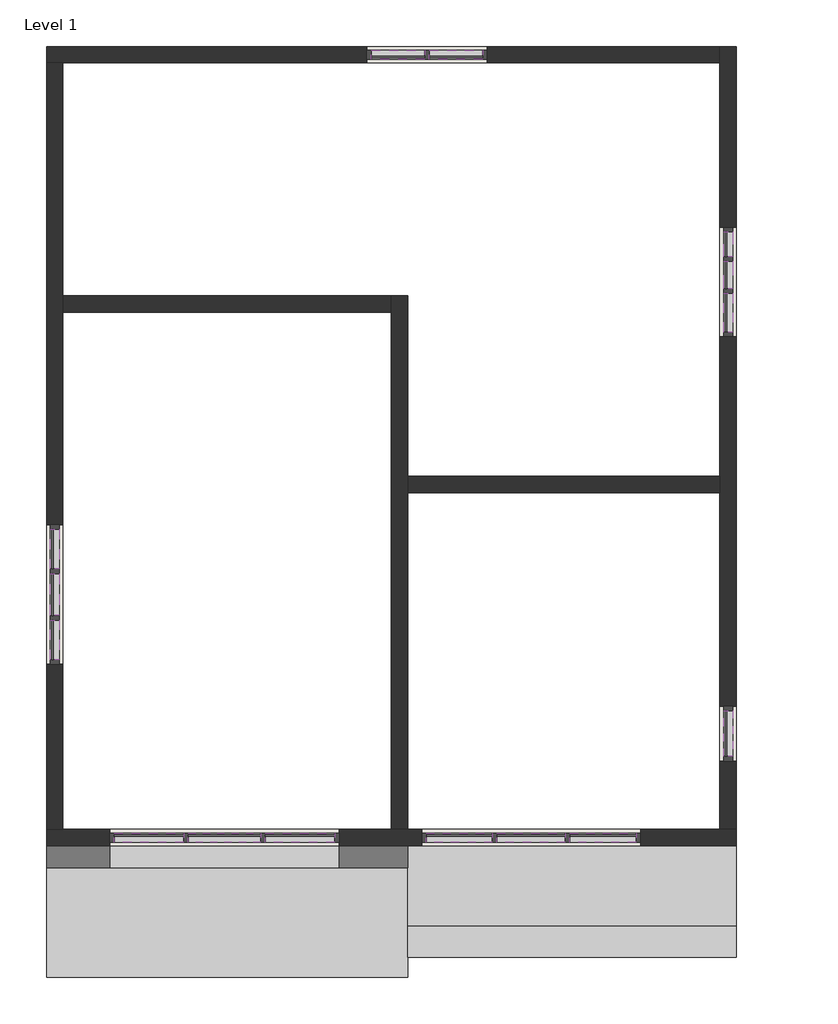
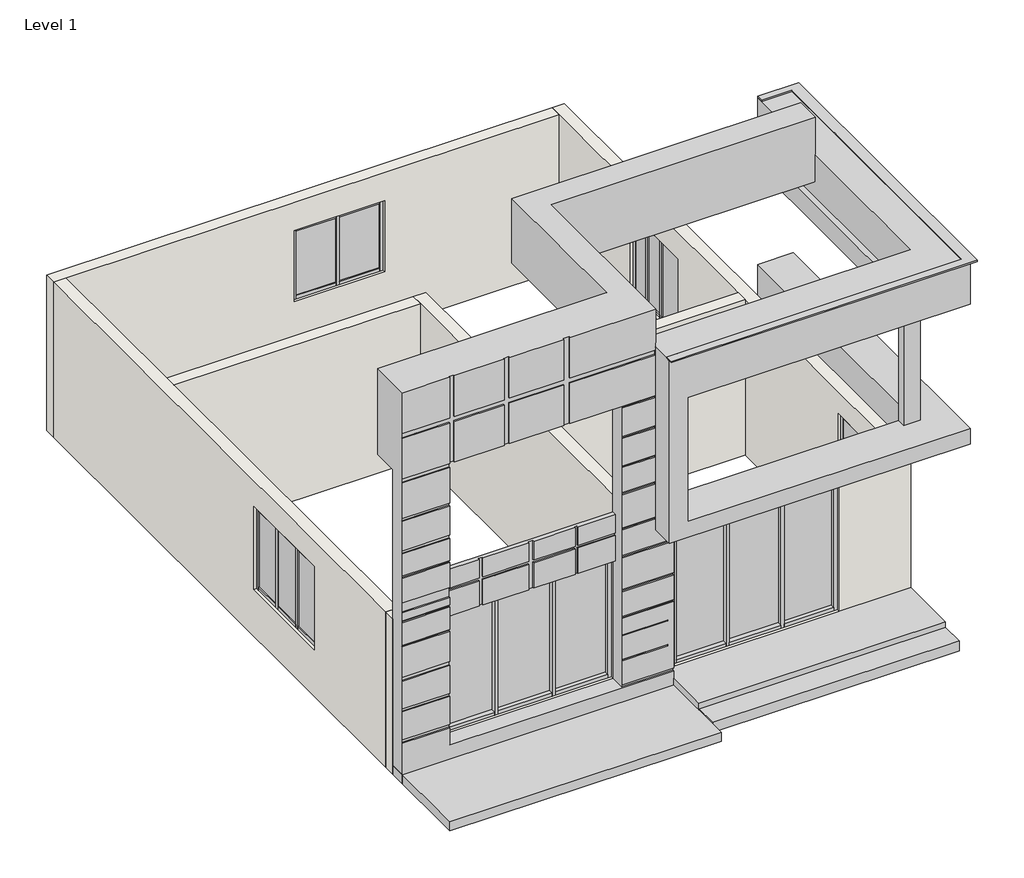
# One storey: 51 members, 15 plates, 7 walls, 3 proxies.
"""IFC4 building model written with IfcOpenShell, lengths in millimetres."""

from ifc_helpers import new_model, si_unit, origin, origin_with_axes, place, context, project, spatial, polyline, outline, extrude, faceted_brep, transform, mapped, element, save
from components import generic_models_1_generic_models_1_2766a2ed, generic_models_2_generic_models_2_78c8f357, generic_models_3_generic_models_3_8fccb6e9, member_801a2072, member_cfcad22e, member_239fd6c5, member_a02723d6, member_ff82125d, member_194e59d8, member_0aac9e43, member_4863f604, member_5e365d0c, member_bb8a6b57, member_285f5b4f, member_dfe75557, member_81de2198, member_e2840d6c, member_3042558b, member_3a0a7659, member_4c2afa05, member_9fe852e5, member_73c075c8, member_623bfa76, member_b1f03c2a, member_3d641c1c, system_panel_glazed_afec1f6d, system_panel_glazed_d4561187, system_panel_glazed_003a5872, system_panel_glazed_ce09be71, system_panel_glazed_e19ac2e9, system_panel_glazed_6b96ba39, system_panel_glazed_232e26bf, system_panel_glazed_d6ecc329, system_panel_glazed_bebac94d, system_panel_glazed_f147d628, system_panel_glazed_06fe117f

model = new_model("IFC4")

# Units and contexts
model_context = context("Model", 3, world=origin())
ifc_project = project(units=[si_unit("LENGTHUNIT", "METRE", prefix="MILLI")], contexts=[model_context])

# Site, building, storey
site = spatial("IfcSite", under=ifc_project)
building = spatial("IfcBuilding", under=site)
storey = spatial("IfcBuildingStorey", under=building, Name="Level 1", Elevation=0.0)

# Proxies
placement = place(None, origin())
generic_models_1_generic_models_1_shape = generic_models_1_generic_models_1_2766a2ed(model_context)
element("IfcBuildingElementProxy", 1, Name="Generic Models 1 : Generic Models 1", ObjectType="Generic Models 1 : Generic Models 1", at=placement, inside=storey, context=model_context, shape_type="MappedRepresentation", body=[
    mapped(generic_models_1_generic_models_1_shape, transform((0.0, 0.0, 0.0), x_axis=(1.0, 0.0, 0.0), y_axis=(0.0, 1.0, 0.0), z_axis=(0.0, 0.0, 1.0))),
])
generic_models_2_generic_models_2_shape = generic_models_2_generic_models_2_78c8f357(model_context)
element("IfcBuildingElementProxy", 2, Name="Generic Models 2 : Generic Models 2", ObjectType="Generic Models 2 : Generic Models 2", at=placement, inside=storey, context=model_context, shape_type="MappedRepresentation", body=[
    mapped(generic_models_2_generic_models_2_shape, transform((0.0, 0.0, 0.0), x_axis=(1.0, 0.0, 0.0), y_axis=(0.0, 1.0, 0.0), z_axis=(0.0, 0.0, 1.0))),
])
generic_models_3_generic_models_3_shape = generic_models_3_generic_models_3_8fccb6e9(model_context)
element("IfcBuildingElementProxy", 3, Name="Generic Models 3 : Generic Models 3", ObjectType="Generic Models 3 : Generic Models 3", at=placement, inside=storey, context=model_context, shape_type="MappedRepresentation", body=[
    mapped(generic_models_3_generic_models_3_shape, transform((0.0, 0.0, 0.0), x_axis=(1.0, 0.0, 0.0), y_axis=(0.0, 1.0, 0.0), z_axis=(0.0, 0.0, 1.0))),
])

# Members
member_shape = member_801a2072(model_context)
element("IfcMember", 4, ObjectType="Rectangular Mullion : 2.5\" x 5\" rectangular", at=placement, inside=storey, context=model_context, shape_type="MappedRepresentation", body=[
    mapped(member_shape, transform((-14543.6018575, -15040.4378384, 458.502719), x_axis=(0.0, 0.0, -1.0), y_axis=(0.0, -1.0, 0.0), z_axis=(-1.0, 0.0, 0.0))),
])
element("IfcMember", 5, ObjectType="Rectangular Mullion : 2.5\" x 5\" rectangular", at=placement, inside=storey, context=model_context, shape_type="MappedRepresentation", body=[
    mapped(member_shape, transform((-16645.4518575, -15040.4378384, 458.502719), x_axis=(0.0, 0.0, -1.0), y_axis=(0.0, -1.0, 0.0), z_axis=(-1.0, 0.0, 0.0))),
])
member_2_shape = member_cfcad22e(model_context)
element("IfcMember", 6, ObjectType="Rectangular Mullion : 2.5\" x 5\" rectangular", at=placement, inside=storey, context=model_context, shape_type="MappedRepresentation", body=[
    mapped(member_2_shape, transform((-15610.4018575, -15040.4378384, 458.502719), x_axis=(0.0, 0.0, -1.0), y_axis=(0.0, -1.0, 0.0), z_axis=(-1.0, 0.0, 0.0))),
])
member_3_shape = member_239fd6c5(model_context)
element("IfcMember", 7, ObjectType="Rectangular Mullion : 2.5\" x 5\" rectangular", at=placement, inside=storey, context=model_context, shape_type="MappedRepresentation", body=[
    mapped(member_3_shape, transform((-15642.1518575, -15040.4378384, 458.502719), x_axis=(1.0, 0.0, 0.0), y_axis=(0.0, -1.0, 0.0), z_axis=(0.0, 0.0, -1.0))),
])
element("IfcMember", 8, ObjectType="Rectangular Mullion : 2.5\" x 5\" rectangular", at=placement, inside=storey, context=model_context, shape_type="MappedRepresentation", body=[
    mapped(member_3_shape, transform((-14575.3518575, -15040.4378384, 458.502719), x_axis=(1.0, 0.0, 0.0), y_axis=(0.0, -1.0, 0.0), z_axis=(0.0, 0.0, -1.0))),
])
element("IfcMember", 9, ObjectType="Rectangular Mullion : 2.5\" x 5\" rectangular", at=placement, inside=storey, context=model_context, shape_type="MappedRepresentation", body=[
    mapped(member_2_shape, transform((-14607.1018575, -15040.4378384, 2802.4335272), x_axis=(0.0, 0.0, 1.0), y_axis=(0.0, -1.0, 0.0), z_axis=(1.0, 0.0, 0.0))),
])
element("IfcMember", 10, ObjectType="Rectangular Mullion : 2.5\" x 5\" rectangular", at=placement, inside=storey, context=model_context, shape_type="MappedRepresentation", body=[
    mapped(member_shape, transform((-15673.9018575, -15040.4378384, 2802.4335272), x_axis=(0.0, 0.0, 1.0), y_axis=(0.0, -1.0, 0.0), z_axis=(1.0, 0.0, 0.0))),
])
element("IfcMember", 11, ObjectType="Rectangular Mullion : 2.5\" x 5\" rectangular", at=placement, inside=storey, context=model_context, shape_type="MappedRepresentation", body=[
    mapped(member_shape, transform((-13572.0518575, -15040.4378384, 2802.4335272), x_axis=(0.0, 0.0, 1.0), y_axis=(0.0, -1.0, 0.0), z_axis=(1.0, 0.0, 0.0))),
])
member_4_shape = member_a02723d6(model_context)
element("IfcMember", 12, ObjectType="Rectangular Mullion : 2.5\" x 5\" rectangular", at=placement, inside=storey, context=model_context, shape_type="MappedRepresentation", body=[
    mapped(member_4_shape, transform((-16708.9518575, -15040.4378384, 2802.4335272), x_axis=(-1.0, 0.0, 0.0), y_axis=(0.0, -1.0, 0.0), z_axis=(0.0, 0.0, 1.0))),
])
element("IfcMember", 13, ObjectType="Rectangular Mullion : 2.5\" x 5\" rectangular", at=placement, inside=storey, context=model_context, shape_type="MappedRepresentation", body=[
    mapped(member_4_shape, transform((-13508.5518575, -15040.4378384, 458.502719), x_axis=(1.0, 0.0, 0.0), y_axis=(0.0, -1.0, 0.0), z_axis=(0.0, 0.0, -1.0))),
])
member_5_shape = member_ff82125d(model_context)
element("IfcMember", 14, ObjectType="Rectangular Mullion : 2.5\" x 5\" rectangular", at=placement, inside=storey, context=model_context, shape_type="MappedRepresentation", body=[
    mapped(member_5_shape, transform((-10301.8018575, -15040.4378384, 304.8), x_axis=(0.0, 0.0, -1.0), y_axis=(0.0, -1.0, 0.0), z_axis=(-1.0, 0.0, 0.0))),
])
element("IfcMember", 15, ObjectType="Rectangular Mullion : 2.5\" x 5\" rectangular", at=placement, inside=storey, context=model_context, shape_type="MappedRepresentation", body=[
    mapped(member_5_shape, transform((-12302.0518575, -15040.4378384, 304.8), x_axis=(0.0, 0.0, -1.0), y_axis=(0.0, -1.0, 0.0), z_axis=(-1.0, 0.0, 0.0))),
])
member_6_shape = member_194e59d8(model_context)
element("IfcMember", 16, ObjectType="Rectangular Mullion : 2.5\" x 5\" rectangular", at=placement, inside=storey, context=model_context, shape_type="MappedRepresentation", body=[
    mapped(member_6_shape, transform((-11317.8018575, -15040.4378384, 304.8), x_axis=(0.0, 0.0, -1.0), y_axis=(0.0, -1.0, 0.0), z_axis=(-1.0, 0.0, 0.0))),
])
member_7_shape = member_0aac9e43(model_context)
element("IfcMember", 17, ObjectType="Rectangular Mullion : 2.5\" x 5\" rectangular", at=placement, inside=storey, context=model_context, shape_type="MappedRepresentation", body=[
    mapped(member_7_shape, transform((-11349.5518575, -15040.4378384, 304.8), x_axis=(1.0, 0.0, 0.0), y_axis=(0.0, -1.0, 0.0), z_axis=(0.0, 0.0, -1.0))),
])
element("IfcMember", 18, ObjectType="Rectangular Mullion : 2.5\" x 5\" rectangular", at=placement, inside=storey, context=model_context, shape_type="MappedRepresentation", body=[
    mapped(member_7_shape, transform((-10333.5518575, -15040.4378384, 304.8), x_axis=(1.0, 0.0, 0.0), y_axis=(0.0, -1.0, 0.0), z_axis=(0.0, 0.0, -1.0))),
])
element("IfcMember", 19, ObjectType="Rectangular Mullion : 2.5\" x 5\" rectangular", at=placement, inside=storey, context=model_context, shape_type="MappedRepresentation", body=[
    mapped(member_6_shape, transform((-10365.3018575, -15040.4378384, 2834.2963211), x_axis=(0.0, 0.0, 1.0), y_axis=(0.0, -1.0, 0.0), z_axis=(1.0, 0.0, 0.0))),
])
element("IfcMember", 20, ObjectType="Rectangular Mullion : 2.5\" x 5\" rectangular", at=placement, inside=storey, context=model_context, shape_type="MappedRepresentation", body=[
    mapped(member_5_shape, transform((-11381.3018575, -15040.4378384, 2834.2963211), x_axis=(0.0, 0.0, 1.0), y_axis=(0.0, -1.0, 0.0), z_axis=(1.0, 0.0, 0.0))),
])
element("IfcMember", 21, ObjectType="Rectangular Mullion : 2.5\" x 5\" rectangular", at=placement, inside=storey, context=model_context, shape_type="MappedRepresentation", body=[
    mapped(member_5_shape, transform((-9381.0518575, -15040.4378384, 2834.2963211), x_axis=(0.0, 0.0, 1.0), y_axis=(0.0, -1.0, 0.0), z_axis=(1.0, 0.0, 0.0))),
])
member_8_shape = member_4863f604(model_context)
element("IfcMember", 22, ObjectType="Rectangular Mullion : 2.5\" x 5\" rectangular", at=placement, inside=storey, context=model_context, shape_type="MappedRepresentation", body=[
    mapped(member_8_shape, transform((-12365.5518575, -15040.4378384, 2834.2963211), x_axis=(-1.0, 0.0, 0.0), y_axis=(0.0, -1.0, 0.0), z_axis=(0.0, 0.0, 1.0))),
])
element("IfcMember", 23, ObjectType="Rectangular Mullion : 2.5\" x 5\" rectangular", at=placement, inside=storey, context=model_context, shape_type="MappedRepresentation", body=[
    mapped(member_8_shape, transform((-9317.5518575, -15040.4378384, 304.8), x_axis=(1.0, 0.0, 0.0), y_axis=(0.0, -1.0, 0.0), z_axis=(0.0, 0.0, -1.0))),
])
member_9_shape = member_5e365d0c(model_context)
element("IfcMember", 24, ObjectType="Rectangular Mullion : 2.5\" x 5\" rectangular", at=placement, inside=storey, context=model_context, shape_type="MappedRepresentation", body=[
    mapped(member_9_shape, transform((-8098.3518575, -13275.1378384, 2614.7944805), x_axis=(0.0, 0.0, 1.0), y_axis=(1.0, 0.0, 0.0), z_axis=(0.0, 1.0, 0.0))),
])
element("IfcMember", 25, ObjectType="Rectangular Mullion : 2.5\" x 5\" rectangular", at=placement, inside=storey, context=model_context, shape_type="MappedRepresentation", body=[
    mapped(member_9_shape, transform((-8098.3518575, -13910.1378384, 626.4916176), x_axis=(0.0, 0.0, -1.0), y_axis=(1.0, 0.0, 0.0), z_axis=(0.0, -1.0, 0.0))),
])
member_10_shape = member_bb8a6b57(model_context)
element("IfcMember", 26, ObjectType="Rectangular Mullion : 2.5\" x 5\" rectangular", at=placement, inside=storey, context=model_context, shape_type="MappedRepresentation", body=[
    mapped(member_10_shape, transform((-8098.3518575, -13211.6378384, 626.4916176), x_axis=(0.0, 1.0, 0.0), y_axis=(1.0, 0.0, 0.0), z_axis=(0.0, 0.0, -1.0))),
])
element("IfcMember", 27, ObjectType="Rectangular Mullion : 2.5\" x 5\" rectangular", at=placement, inside=storey, context=model_context, shape_type="MappedRepresentation", body=[
    mapped(member_10_shape, transform((-8098.3518575, -13973.6378384, 2614.7944805), x_axis=(0.0, -1.0, 0.0), y_axis=(1.0, 0.0, 0.0), z_axis=(0.0, 0.0, 1.0))),
])
member_11_shape = member_285f5b4f(model_context)
element("IfcMember", 28, ObjectType="Rectangular Mullion : 2.5\" x 5\" rectangular", at=placement, inside=storey, context=model_context, shape_type="MappedRepresentation", body=[
    mapped(member_11_shape, transform((-8098.3518575, -6956.8878384, 948.2533356), x_axis=(0.0, 0.0, -1.0), y_axis=(1.0, 0.0, 0.0), z_axis=(0.0, -1.0, 0.0))),
])
member_12_shape = member_dfe75557(model_context)
element("IfcMember", 29, ObjectType="Rectangular Mullion : 2.5\" x 5\" rectangular", at=placement, inside=storey, context=model_context, shape_type="MappedRepresentation", body=[
    mapped(member_12_shape, transform((-8098.3518575, -7401.3878384, 948.2533356), x_axis=(0.0, 0.0, -1.0), y_axis=(1.0, 0.0, 0.0), z_axis=(0.0, -1.0, 0.0))),
])
member_13_shape = member_81de2198(model_context)
element("IfcMember", 30, ObjectType="Rectangular Mullion : 2.5\" x 5\" rectangular", at=placement, inside=storey, context=model_context, shape_type="MappedRepresentation", body=[
    mapped(member_13_shape, transform((-8098.3518575, -8004.6378384, 948.2533356), x_axis=(0.0, 0.0, -1.0), y_axis=(1.0, 0.0, 0.0), z_axis=(0.0, -1.0, 0.0))),
])
member_14_shape = member_e2840d6c(model_context)
element("IfcMember", 31, ObjectType="Rectangular Mullion : 2.5\" x 5\" rectangular", at=placement, inside=storey, context=model_context, shape_type="MappedRepresentation", body=[
    mapped(member_14_shape, transform((-8098.3518575, -7433.1378384, 948.2533356), x_axis=(0.0, 1.0, 0.0), y_axis=(1.0, 0.0, 0.0), z_axis=(0.0, 0.0, -1.0))),
])
element("IfcMember", 32, ObjectType="Rectangular Mullion : 2.5\" x 5\" rectangular", at=placement, inside=storey, context=model_context, shape_type="MappedRepresentation", body=[
    mapped(member_14_shape, transform((-8098.3518575, -6988.6378384, 948.2533356), x_axis=(0.0, 1.0, 0.0), y_axis=(1.0, 0.0, 0.0), z_axis=(0.0, 0.0, -1.0))),
])
element("IfcMember", 33, ObjectType="Rectangular Mullion : 2.5\" x 5\" rectangular", at=placement, inside=storey, context=model_context, shape_type="MappedRepresentation", body=[
    mapped(member_12_shape, transform((-8098.3518575, -7020.3878384, 2528.306786), x_axis=(0.0, 0.0, 1.0), y_axis=(1.0, 0.0, 0.0), z_axis=(0.0, 1.0, 0.0))),
])
element("IfcMember", 34, ObjectType="Rectangular Mullion : 2.5\" x 5\" rectangular", at=placement, inside=storey, context=model_context, shape_type="MappedRepresentation", body=[
    mapped(member_13_shape, transform((-8098.3518575, -7464.8878384, 2528.306786), x_axis=(0.0, 0.0, 1.0), y_axis=(1.0, 0.0, 0.0), z_axis=(0.0, 1.0, 0.0))),
])
element("IfcMember", 35, ObjectType="Rectangular Mullion : 2.5\" x 5\" rectangular", at=placement, inside=storey, context=model_context, shape_type="MappedRepresentation", body=[
    mapped(member_11_shape, transform((-8098.3518575, -6607.6378384, 2528.306786), x_axis=(0.0, 0.0, 1.0), y_axis=(1.0, 0.0, 0.0), z_axis=(0.0, 1.0, 0.0))),
])
member_15_shape = member_3042558b(model_context)
element("IfcMember", 36, ObjectType="Rectangular Mullion : 2.5\" x 5\" rectangular", at=placement, inside=storey, context=model_context, shape_type="MappedRepresentation", body=[
    mapped(member_15_shape, transform((-8098.3518575, -6544.1378384, 948.2533356), x_axis=(0.0, 1.0, 0.0), y_axis=(1.0, 0.0, 0.0), z_axis=(0.0, 0.0, -1.0))),
])
element("IfcMember", 37, ObjectType="Rectangular Mullion : 2.5\" x 5\" rectangular", at=placement, inside=storey, context=model_context, shape_type="MappedRepresentation", body=[
    mapped(member_15_shape, transform((-8098.3518575, -8068.1378384, 2528.306786), x_axis=(0.0, -1.0, 0.0), y_axis=(1.0, 0.0, 0.0), z_axis=(0.0, 0.0, 1.0))),
])
member_16_shape = member_3a0a7659(model_context)
element("IfcMember", 38, ObjectType="Rectangular Mullion : 2.5\" x 5\" rectangular", at=placement, inside=storey, context=model_context, shape_type="MappedRepresentation", body=[
    mapped(member_16_shape, transform((-12257.6018575, -4143.8378384, 2493.273831), x_axis=(0.0, 0.0, 1.0), y_axis=(0.0, 1.0, 0.0), z_axis=(-1.0, 0.0, 0.0))),
])
element("IfcMember", 39, ObjectType="Rectangular Mullion : 2.5\" x 5\" rectangular", at=placement, inside=storey, context=model_context, shape_type="MappedRepresentation", body=[
    mapped(member_16_shape, transform((-13064.0518575, -4143.8378384, 2493.273831), x_axis=(0.0, 0.0, 1.0), y_axis=(0.0, 1.0, 0.0), z_axis=(-1.0, 0.0, 0.0))),
])
element("IfcMember", 40, ObjectType="Rectangular Mullion : 2.5\" x 5\" rectangular", at=placement, inside=storey, context=model_context, shape_type="MappedRepresentation", body=[
    mapped(member_16_shape, transform((-12321.1018575, -4143.8378384, 1101.8659171), x_axis=(0.0, 0.0, -1.0), y_axis=(0.0, 1.0, 0.0), z_axis=(1.0, 0.0, 0.0))),
])
element("IfcMember", 41, ObjectType="Rectangular Mullion : 2.5\" x 5\" rectangular", at=placement, inside=storey, context=model_context, shape_type="MappedRepresentation", body=[
    mapped(member_16_shape, transform((-11514.6518575, -4143.8378384, 1101.8659171), x_axis=(0.0, 0.0, -1.0), y_axis=(0.0, 1.0, 0.0), z_axis=(1.0, 0.0, 0.0))),
])
member_17_shape = member_4c2afa05(model_context)
element("IfcMember", 42, ObjectType="Rectangular Mullion : 2.5\" x 5\" rectangular", at=placement, inside=storey, context=model_context, shape_type="MappedRepresentation", body=[
    mapped(member_17_shape, transform((-12289.3518575, -4143.8378384, 1101.8659171), x_axis=(-1.0, 0.0, 0.0), y_axis=(0.0, 1.0, 0.0), z_axis=(0.0, 0.0, -1.0))),
])
member_18_shape = member_9fe852e5(model_context)
element("IfcMember", 43, ObjectType="Rectangular Mullion : 2.5\" x 5\" rectangular", at=placement, inside=storey, context=model_context, shape_type="MappedRepresentation", body=[
    mapped(member_18_shape, transform((-11451.1518575, -4143.8378384, 2493.273831), x_axis=(1.0, 0.0, 0.0), y_axis=(0.0, 1.0, 0.0), z_axis=(0.0, 0.0, 1.0))),
])
element("IfcMember", 44, ObjectType="Rectangular Mullion : 2.5\" x 5\" rectangular", at=placement, inside=storey, context=model_context, shape_type="MappedRepresentation", body=[
    mapped(member_18_shape, transform((-13127.5518575, -4143.8378384, 1101.8659171), x_axis=(-1.0, 0.0, 0.0), y_axis=(0.0, 1.0, 0.0), z_axis=(0.0, 0.0, -1.0))),
])
member_19_shape = member_73c075c8(model_context)
element("IfcMember", 45, ObjectType="Rectangular Mullion : 2.5\" x 5\" rectangular", at=placement, inside=storey, context=model_context, shape_type="MappedRepresentation", body=[
    mapped(member_19_shape, transform((-17470.9518575, -11300.2878384, 914.5062999), x_axis=(0.0, 0.0, -1.0), y_axis=(1.0, 0.0, 0.0), z_axis=(0.0, -1.0, 0.0))),
])
element("IfcMember", 46, ObjectType="Rectangular Mullion : 2.5\" x 5\" rectangular", at=placement, inside=storey, context=model_context, shape_type="MappedRepresentation", body=[
    mapped(member_19_shape, transform((-17470.9518575, -12563.9378384, 914.5062999), x_axis=(0.0, 0.0, -1.0), y_axis=(1.0, 0.0, 0.0), z_axis=(0.0, -1.0, 0.0))),
])
member_20_shape = member_623bfa76(model_context)
element("IfcMember", 47, ObjectType="Rectangular Mullion : 2.5\" x 5\" rectangular", at=placement, inside=storey, context=model_context, shape_type="MappedRepresentation", body=[
    mapped(member_20_shape, transform((-17470.9518575, -11947.9878384, 914.5062999), x_axis=(0.0, 0.0, -1.0), y_axis=(1.0, 0.0, 0.0), z_axis=(0.0, -1.0, 0.0))),
])
member_21_shape = member_b1f03c2a(model_context)
element("IfcMember", 48, ObjectType="Rectangular Mullion : 2.5\" x 5\" rectangular", at=placement, inside=storey, context=model_context, shape_type="MappedRepresentation", body=[
    mapped(member_21_shape, transform((-17470.9518575, -11332.0378384, 914.5062999), x_axis=(0.0, 1.0, 0.0), y_axis=(1.0, 0.0, 0.0), z_axis=(0.0, 0.0, -1.0))),
])
element("IfcMember", 49, ObjectType="Rectangular Mullion : 2.5\" x 5\" rectangular", at=placement, inside=storey, context=model_context, shape_type="MappedRepresentation", body=[
    mapped(member_21_shape, transform((-17470.9518575, -11979.7378384, 914.5062999), x_axis=(0.0, 1.0, 0.0), y_axis=(1.0, 0.0, 0.0), z_axis=(0.0, 0.0, -1.0))),
])
element("IfcMember", 50, ObjectType="Rectangular Mullion : 2.5\" x 5\" rectangular", at=placement, inside=storey, context=model_context, shape_type="MappedRepresentation", body=[
    mapped(member_20_shape, transform((-17470.9518575, -11363.7878384, 2543.5318085), x_axis=(0.0, 0.0, 1.0), y_axis=(1.0, 0.0, 0.0), z_axis=(0.0, 1.0, 0.0))),
])
element("IfcMember", 51, ObjectType="Rectangular Mullion : 2.5\" x 5\" rectangular", at=placement, inside=storey, context=model_context, shape_type="MappedRepresentation", body=[
    mapped(member_19_shape, transform((-17470.9518575, -12011.4878384, 2543.5318085), x_axis=(0.0, 0.0, 1.0), y_axis=(1.0, 0.0, 0.0), z_axis=(0.0, 1.0, 0.0))),
])
element("IfcMember", 52, ObjectType="Rectangular Mullion : 2.5\" x 5\" rectangular", at=placement, inside=storey, context=model_context, shape_type="MappedRepresentation", body=[
    mapped(member_19_shape, transform((-17470.9518575, -10747.8378384, 2543.5318085), x_axis=(0.0, 0.0, 1.0), y_axis=(1.0, 0.0, 0.0), z_axis=(0.0, 1.0, 0.0))),
])
member_22_shape = member_3d641c1c(model_context)
element("IfcMember", 53, ObjectType="Rectangular Mullion : 2.5\" x 5\" rectangular", at=placement, inside=storey, context=model_context, shape_type="MappedRepresentation", body=[
    mapped(member_22_shape, transform((-17470.9518575, -10684.3378384, 914.5062999), x_axis=(0.0, 1.0, 0.0), y_axis=(1.0, 0.0, 0.0), z_axis=(0.0, 0.0, -1.0))),
])
element("IfcMember", 54, ObjectType="Rectangular Mullion : 2.5\" x 5\" rectangular", at=placement, inside=storey, context=model_context, shape_type="MappedRepresentation", body=[
    mapped(member_22_shape, transform((-17470.9518575, -12627.4378384, 2543.5318085), x_axis=(0.0, -1.0, 0.0), y_axis=(1.0, 0.0, 0.0), z_axis=(0.0, 0.0, 1.0))),
])

# Plates
system_panel_glazed_shape = system_panel_glazed_afec1f6d(model_context)
element("IfcPlate", 55, ObjectType="System Panel : Glazed", at=placement, inside=storey, context=model_context, shape_type="MappedRepresentation", body=[
    mapped(system_panel_glazed_shape, transform((-16159.6768575, -15040.4378384, 522.002719), x_axis=(1.0, 0.0, 0.0), y_axis=(0.0, 1.0, 0.0), z_axis=(0.0, 0.0, 1.0))),
])
element("IfcPlate", 56, ObjectType="System Panel : Glazed", at=placement, inside=storey, context=model_context, shape_type="MappedRepresentation", body=[
    mapped(system_panel_glazed_shape, transform((-14057.8268575, -15040.4378384, 522.002719), x_axis=(1.0, 0.0, 0.0), y_axis=(0.0, 1.0, 0.0), z_axis=(0.0, 0.0, 1.0))),
])
system_panel_glazed_2_shape = system_panel_glazed_d4561187(model_context)
element("IfcPlate", 57, ObjectType="System Panel : Glazed", at=placement, inside=storey, context=model_context, shape_type="MappedRepresentation", body=[
    mapped(system_panel_glazed_2_shape, transform((-15108.7518575, -15040.4378384, 522.002719), x_axis=(1.0, 0.0, 0.0), y_axis=(0.0, 1.0, 0.0), z_axis=(0.0, 0.0, 1.0))),
])
system_panel_glazed_3_shape = system_panel_glazed_003a5872(model_context)
element("IfcPlate", 58, ObjectType="System Panel : Glazed", at=placement, inside=storey, context=model_context, shape_type="MappedRepresentation", body=[
    mapped(system_panel_glazed_3_shape, transform((-11841.6768575, -15040.4378384, 368.3), x_axis=(1.0, 0.0, 0.0), y_axis=(0.0, 1.0, 0.0), z_axis=(0.0, 0.0, 1.0))),
])
element("IfcPlate", 59, ObjectType="System Panel : Glazed", at=placement, inside=storey, context=model_context, shape_type="MappedRepresentation", body=[
    mapped(system_panel_glazed_3_shape, transform((-9841.4268575, -15040.4378384, 368.3), x_axis=(1.0, 0.0, 0.0), y_axis=(0.0, 1.0, 0.0), z_axis=(0.0, 0.0, 1.0))),
])
system_panel_glazed_4_shape = system_panel_glazed_ce09be71(model_context)
element("IfcPlate", 60, ObjectType="System Panel : Glazed", at=placement, inside=storey, context=model_context, shape_type="MappedRepresentation", body=[
    mapped(system_panel_glazed_4_shape, transform((-10841.5518575, -15040.4378384, 368.3), x_axis=(1.0, 0.0, 0.0), y_axis=(0.0, 1.0, 0.0), z_axis=(0.0, 0.0, 1.0))),
])
system_panel_glazed_5_shape = system_panel_glazed_e19ac2e9(model_context)
element("IfcPlate", 61, ObjectType="System Panel : Glazed", at=placement, inside=storey, context=model_context, shape_type="MappedRepresentation", body=[
    mapped(system_panel_glazed_5_shape, transform((-8098.3518575, -13592.6378384, 689.9916176), x_axis=(0.0, 1.0, 0.0), y_axis=(-1.0, 0.0, 0.0), z_axis=(0.0, 0.0, 1.0))),
])
system_panel_glazed_6_shape = system_panel_glazed_6b96ba39(model_context)
element("IfcPlate", 62, ObjectType="System Panel : Glazed", at=placement, inside=storey, context=model_context, shape_type="MappedRepresentation", body=[
    mapped(system_panel_glazed_6_shape, transform((-8098.3518575, -7734.7628384, 1011.7533356), x_axis=(0.0, 1.0, 0.0), y_axis=(-1.0, 0.0, 0.0), z_axis=(0.0, 0.0, 1.0))),
])
system_panel_glazed_7_shape = system_panel_glazed_232e26bf(model_context)
element("IfcPlate", 63, ObjectType="System Panel : Glazed", at=placement, inside=storey, context=model_context, shape_type="MappedRepresentation", body=[
    mapped(system_panel_glazed_7_shape, transform((-8098.3518575, -7210.8878384, 1011.7533356), x_axis=(0.0, 1.0, 0.0), y_axis=(-1.0, 0.0, 0.0), z_axis=(0.0, 0.0, 1.0))),
])
system_panel_glazed_8_shape = system_panel_glazed_d6ecc329(model_context)
element("IfcPlate", 64, ObjectType="System Panel : Glazed", at=placement, inside=storey, context=model_context, shape_type="MappedRepresentation", body=[
    mapped(system_panel_glazed_8_shape, transform((-8098.3518575, -6782.2628384, 1011.7533356), x_axis=(0.0, 1.0, 0.0), y_axis=(-1.0, 0.0, 0.0), z_axis=(0.0, 0.0, 1.0))),
])
system_panel_glazed_9_shape = system_panel_glazed_bebac94d(model_context)
element("IfcPlate", 65, ObjectType="System Panel : Glazed", at=placement, inside=storey, context=model_context, shape_type="MappedRepresentation", body=[
    mapped(system_panel_glazed_9_shape, transform((-11886.1268575, -4143.8378384, 1165.3659171), x_axis=(-1.0, 0.0, 0.0), y_axis=(0.0, -1.0, 0.0), z_axis=(0.0, 0.0, 1.0))),
])
element("IfcPlate", 66, ObjectType="System Panel : Glazed", at=placement, inside=storey, context=model_context, shape_type="MappedRepresentation", body=[
    mapped(system_panel_glazed_9_shape, transform((-12692.5768575, -4143.8378384, 1165.3659171), x_axis=(-1.0, 0.0, 0.0), y_axis=(0.0, -1.0, 0.0), z_axis=(0.0, 0.0, 1.0))),
])
system_panel_glazed_10_shape = system_panel_glazed_f147d628(model_context)
element("IfcPlate", 67, ObjectType="System Panel : Glazed", at=placement, inside=storey, context=model_context, shape_type="MappedRepresentation", body=[
    mapped(system_panel_glazed_10_shape, transform((-17470.9518575, -12287.7128384, 978.0062999), x_axis=(0.0, 1.0, 0.0), y_axis=(-1.0, 0.0, 0.0), z_axis=(0.0, 0.0, 1.0))),
])
element("IfcPlate", 68, ObjectType="System Panel : Glazed", at=placement, inside=storey, context=model_context, shape_type="MappedRepresentation", body=[
    mapped(system_panel_glazed_10_shape, transform((-17470.9518575, -11024.0628384, 978.0062999), x_axis=(0.0, 1.0, 0.0), y_axis=(-1.0, 0.0, 0.0), z_axis=(0.0, 0.0, 1.0))),
])
system_panel_glazed_11_shape = system_panel_glazed_06fe117f(model_context)
element("IfcPlate", 69, ObjectType="System Panel : Glazed", at=placement, inside=storey, context=model_context, shape_type="MappedRepresentation", body=[
    mapped(system_panel_glazed_11_shape, transform((-17470.9518575, -11655.8878384, 978.0062999), x_axis=(0.0, 1.0, 0.0), y_axis=(-1.0, 0.0, 0.0), z_axis=(0.0, 0.0, 1.0))),
])

# Walls
element("IfcWall", 70, ObjectType="9\"", at=placement, inside=storey, context=model_context, shape_type="Brep", body=[
    faceted_brep([(-17585.2518575, -15154.7378384, 0.0), (-7984.0518575, -15154.7378384, 0.0), (-7984.0518575, -15154.7378384, 3048.0), (-17585.2518575, -15154.7378384, 3048.0), (-12365.5518575, -15154.7378384, 304.8), (-12365.5518575, -15154.7378384, 2834.2963211), (-9317.5518575, -15154.7378384, 2834.2963211), (-9317.5518575, -15154.7378384, 304.8), (-16708.9518575, -15154.7378384, 458.502719), (-16708.9518575, -15154.7378384, 2802.4335272), (-13508.5518575, -15154.7378384, 2802.4335272), (-13508.5518575, -15154.7378384, 458.502719), (-7984.0518575, -14926.1378384, 0.0), (-8212.6518575, -14926.1378384, 0.0), (-12556.0518575, -14926.1378384, 0.0), (-12784.6518575, -14926.1378384, 0.0), (-17356.6518575, -14926.1378384, 0.0), (-17585.2518575, -14926.1378384, 0.0), (-17585.2518575, -14926.1378384, 3048.0), (-17356.6518575, -14926.1378384, 3048.0), (-12784.6518575, -14926.1378384, 3048.0), (-12556.0518575, -14926.1378384, 3048.0), (-8212.6518575, -14926.1378384, 3048.0), (-7984.0518575, -14926.1378384, 3048.0), (-12365.5518575, -14926.1378384, 2834.2963211), (-12365.5518575, -14926.1378384, 304.8), (-9317.5518575, -14926.1378384, 304.8), (-9317.5518575, -14926.1378384, 2834.2963211), (-16708.9518575, -14926.1378384, 2802.4335272), (-16708.9518575, -14926.1378384, 458.502719), (-13508.5518575, -14926.1378384, 458.502719), (-13508.5518575, -14926.1378384, 2802.4335272)], [[[0, 1, 2, 3], [4, 5, 6, 7], [8, 9, 10, 11]], [[12, 13, 14, 15, 16, 17, 18, 19, 20, 21, 22, 23], [24, 25, 26, 27], [28, 29, 30, 31]], [[1, 0, 17, 16, 15, 14, 13, 12]], [[3, 2, 23, 22, 21, 20, 19, 18]], [[2, 1, 12, 23]], [[0, 3, 18, 17]], [[4, 25, 24, 5]], [[5, 24, 27, 6]], [[6, 27, 26, 7]], [[25, 4, 7, 26]], [[28, 9, 8, 29]], [[9, 28, 31, 10]], [[10, 31, 30, 11]], [[29, 8, 11, 30]]]),
])
element("IfcWall", 71, ObjectType="9\"", at=placement, inside=storey, context=model_context, shape_type="Brep", body=[
    faceted_brep([(-7984.0518575, -14926.1378384, 0.0), (-7984.0518575, -4029.5378384, 0.0), (-7984.0518575, -4029.5378384, 3048.0), (-7984.0518575, -14926.1378384, 3048.0), (-7984.0518575, -13973.6378384, 626.4916176), (-7984.0518575, -13973.6378384, 2614.7944805), (-7984.0518575, -13211.6378384, 2614.7944805), (-7984.0518575, -13211.6378384, 626.4916176), (-7984.0518575, -8068.1378384, 948.2533356), (-7984.0518575, -8068.1378384, 2528.306786), (-7984.0518575, -6544.1378384, 2528.306786), (-7984.0518575, -6544.1378384, 948.2533356), (-8212.6518575, -4029.5378384, 0.0), (-8212.6518575, -4258.1378384, 0.0), (-8212.6518575, -10011.2378384, 0.0), (-8212.6518575, -10239.8378384, 0.0), (-8212.6518575, -14926.1378384, 0.0), (-8212.6518575, -14926.1378384, 3048.0), (-8212.6518575, -10239.8378384, 3048.0), (-8212.6518575, -10011.2378384, 3048.0), (-8212.6518575, -4258.1378384, 3048.0), (-8212.6518575, -4029.5378384, 3048.0), (-8212.6518575, -13973.6378384, 2614.7944805), (-8212.6518575, -13973.6378384, 626.4916176), (-8212.6518575, -13211.6378384, 626.4916176), (-8212.6518575, -13211.6378384, 2614.7944805), (-8212.6518575, -8068.1378384, 2528.306786), (-8212.6518575, -8068.1378384, 948.2533356), (-8212.6518575, -6544.1378384, 948.2533356), (-8212.6518575, -6544.1378384, 2528.306786)], [[[0, 1, 2, 3], [4, 5, 6, 7], [8, 9, 10, 11]], [[12, 13, 14, 15, 16, 17, 18, 19, 20, 21], [22, 23, 24, 25], [26, 27, 28, 29]], [[1, 0, 16, 15, 14, 13, 12]], [[3, 2, 21, 20, 19, 18, 17]], [[0, 3, 17, 16]], [[2, 1, 12, 21]], [[4, 23, 22, 5]], [[5, 22, 25, 6]], [[6, 25, 24, 7]], [[23, 4, 7, 24]], [[8, 27, 26, 9]], [[9, 26, 29, 10]], [[28, 11, 10, 29]], [[27, 8, 11, 28]]]),
])
element("IfcWall", 72, ObjectType="9\"", at=placement, inside=storey, context=model_context, shape_type="Brep", body=[
    faceted_brep([(-8212.6518575, -4029.5378384, 0.0), (-17585.2518575, -4029.5378384, 0.0), (-17585.2518575, -4029.5378384, 3048.0), (-8212.6518575, -4029.5378384, 3048.0), (-11451.1518575, -4029.5378384, 1101.8659171), (-11451.1518575, -4029.5378384, 2493.273831), (-13127.5518575, -4029.5378384, 2493.273831), (-13127.5518575, -4029.5378384, 1101.8659171), (-17585.2518575, -4258.1378384, 0.0), (-17356.6518575, -4258.1378384, 0.0), (-8212.6518575, -4258.1378384, 0.0), (-8212.6518575, -4258.1378384, 3048.0), (-17356.6518575, -4258.1378384, 3048.0), (-17585.2518575, -4258.1378384, 3048.0), (-11451.1518575, -4258.1378384, 2493.273831), (-11451.1518575, -4258.1378384, 1101.8659171), (-13127.5518575, -4258.1378384, 1101.8659171), (-13127.5518575, -4258.1378384, 2493.273831)], [[[0, 1, 2, 3], [4, 5, 6, 7]], [[8, 9, 10, 11, 12, 13], [14, 15, 16, 17]], [[1, 0, 10, 9, 8]], [[3, 2, 13, 12, 11]], [[0, 3, 11, 10]], [[2, 1, 8, 13]], [[4, 15, 14, 5]], [[5, 14, 17, 6]], [[6, 17, 16, 7]], [[15, 4, 7, 16]]]),
])
element("IfcWall", 73, ObjectType="9\"", at=placement, inside=storey, context=model_context, shape_type="Brep", body=[
    faceted_brep([(-17585.2518575, -4258.1378384, 0.0), (-17585.2518575, -14926.1378384, 0.0), (-17585.2518575, -14926.1378384, 3048.0), (-17585.2518575, -4258.1378384, 3048.0), (-17585.2518575, -12627.4378384, 2543.5318085), (-17585.2518575, -12627.4378384, 914.5062999), (-17585.2518575, -10684.3378384, 914.5062999), (-17585.2518575, -10684.3378384, 2543.5318085), (-17356.6518575, -14926.1378384, 0.0), (-17356.6518575, -7725.2378384, 0.0), (-17356.6518575, -7496.6378384, 0.0), (-17356.6518575, -4258.1378384, 0.0), (-17356.6518575, -4258.1378384, 3048.0), (-17356.6518575, -7496.6378384, 3048.0), (-17356.6518575, -7725.2378384, 3048.0), (-17356.6518575, -14926.1378384, 3048.0), (-17356.6518575, -12627.4378384, 914.5062999), (-17356.6518575, -12627.4378384, 2543.5318085), (-17356.6518575, -10684.3378384, 2543.5318085), (-17356.6518575, -10684.3378384, 914.5062999)], [[[0, 1, 2, 3], [4, 5, 6, 7]], [[8, 9, 10, 11, 12, 13, 14, 15], [16, 17, 18, 19]], [[1, 0, 11, 10, 9, 8]], [[3, 2, 15, 14, 13, 12]], [[0, 3, 12, 11]], [[2, 1, 8, 15]], [[16, 5, 4, 17]], [[17, 4, 7, 18]], [[18, 7, 6, 19]], [[5, 16, 19, 6]]]),
])
element("IfcWall", 74, ObjectType="9\"", at=placement, inside=storey, context=model_context, shape_type="Brep", body=[
    faceted_brep([(-12556.0518575, -14926.1378384, 0.0), (-12556.0518575, -10239.8378384, 0.0), (-12556.0518575, -10011.2378384, 0.0), (-12556.0518575, -7496.6378384, 0.0), (-12556.0518575, -7496.6378384, 3048.0), (-12556.0518575, -10011.2378384, 3048.0), (-12556.0518575, -10239.8378384, 3048.0), (-12556.0518575, -14926.1378384, 3048.0), (-12784.6518575, -14926.1378384, 0.0), (-12784.6518575, -14926.1378384, 3048.0), (-12784.6518575, -7725.2378384, 3048.0), (-12784.6518575, -7496.6378384, 3048.0), (-12784.6518575, -7496.6378384, 0.0), (-12784.6518575, -7725.2378384, 0.0)], [[[0, 1, 2, 3, 4, 5, 6, 7]], [[8, 9, 10, 11, 12, 13]], [[3, 2, 1, 0, 8, 13, 12]], [[7, 6, 5, 4, 11, 10, 9]], [[0, 7, 9, 8]], [[4, 3, 12, 11]]]),
])
element("IfcWall", 75, ObjectType="9\"", at=placement, inside=storey, context=model_context, shape_type="SweptSolid", body=[
    extrude(outline(polyline([(-8212.6518575, -10239.8378384), (-12556.0518575, -10239.8378384), (-12556.0518575, -10011.2378384), (-8212.6518575, -10011.2378384), (-8212.6518575, -10239.8378384)])), origin_with_axes(), (0.0, 0.0, 1.0), 3048.0),
])
element("IfcWall", 76, ObjectType="9\"", at=placement, inside=storey, context=model_context, shape_type="SweptSolid", body=[
    extrude(outline(polyline([(-17356.6518575, -7496.6378384), (-12784.6518575, -7496.6378384), (-12784.6518575, -7725.2378384), (-17356.6518575, -7725.2378384), (-17356.6518575, -7496.6378384)])), origin_with_axes(), (0.0, 0.0, 1.0), 3048.0),
])

save(model, "model.ifc")

# Revit data of these elements
# Type "Rectangular Mullion : 2.5\" x 5\" rectangular"
#   built-in parameter 1007304 = 0.416667 (stored number, unit not read)
#   built-in parameter 1007301 = 0.104167 (stored number, unit not read)
#   built-in parameter 1007300 = 0.104167 (stored number, unit not read)
# Type "System Panel : Glazed"
#   Construction Type Id = "GSP4R"
#   Analytic Construction = "1/8 in Pilkington single glazing"
#   Visual Light Transmittance = 0.9
#   Solar Heat Gain Coefficient = 0.86
#   Heat Transfer Coefficient (U) = 1.18115 BTU/(h·ft²·°F)
#   Define Thermal Properties by = 1
# Type "9\""
#   Assembly Code = "B2010"
#   Layers, outside or top first: 0' - 9" no material (function 1)
# Element 1 (IfcBuildingElementProxy, "Generic Models 1 : Generic Models 1")
#   Phase Created = New Construction
# Element 2 (IfcBuildingElementProxy, "Generic Models 2 : Generic Models 2")
#   Phase Created = New Construction
# Element 3 (IfcBuildingElementProxy, "Generic Models 3 : Generic Models 3")
#   Phase Created = New Construction
# Elements 4, 5, 6, 7, 8, 9, 10, 11, 12, 13, 14, 15, 16, 17, 18, 19, 20, 21, 22, 23, 24, 25, 26, 27, 28, 29, 30, 31, 32, 33, 34, 35, 36, 37, 38, 39, 40, 41, 42, 43, 44, 45, 46, 47, 48, 49, 50, 51, 52, 53, 54 (IfcMember, "Rectangular Mullion : 2.5\" x 5\" rectangular")
#   Phase Created = New Construction
#   Materials on its faces: "Aluminum"
# Elements 55, 56, 57, 58, 59, 60, 61, 62, 63, 64, 65, 66, 67, 68, 69 (IfcPlate, "System Panel : Glazed")
#   Phase Created = New Construction
#   Materials on its faces: "Glass"
# Elements 70, 71, 72, 73, 74, 75, 76 (IfcWall, "9\"")
#   Top Offset = 0' - 0"
#   Base Offset = 0' - 0"
#   Unconnected Height = 10' - 0"
#   wall height = 10' - 0"
#   Phase Created = New Construction
#   Base Constraint = Level 1
#   Materials on its faces: "Default Wall"
# Materials
#   "Aluminum": class "Metal", colour RGB 247 247 247, transparency 0, Description = "Aluminum 6061", Cost = 0
#   "Glass": class "Glass", colour RGB 0 128 192, transparency 0.75, Description = "Soda Lime Glass", Cost = 0
#   "Default Wall": colour RGB 128 128 128, transparency 0, Cost = 0
